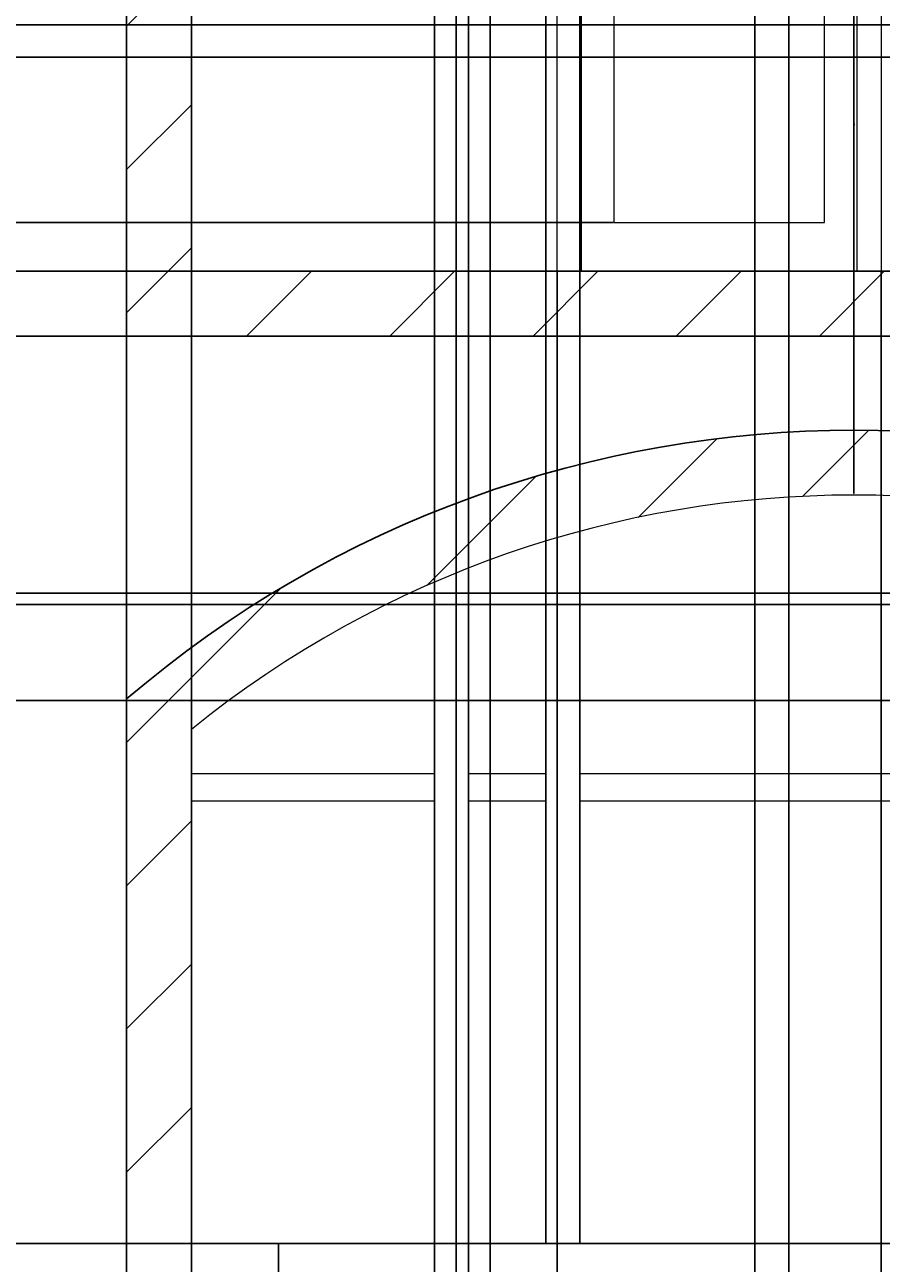
# Model space of a CAD drawing. Units: inches. Extents: x -14 to 375, y -86 to 549.
# Tile 3 of 12: x 122 to 227, y 4 to 156. Entities that reach past the tile are written whole.
import ezdxf

# ---------------------------------------------------------------- set-up
doc = ezdxf.new("R2010")
doc.units = ezdxf.units.IN
doc.header["$MEASUREMENT"] = 0
for name, color, linetype, lineweight in [('A-ANNO-DIMS', 2, 'Continuous', 18), ('A-DOOR', 3, 'Continuous', 18), ('A-ELEV', 7, 'Continuous', 25), ('A-ELEV-PATT', 8, 'Continuous', 13), ('A-GLAZ', 4, 'Continuous', 18)]:
    doc.layers.add(name, color=color, linetype=linetype, lineweight=lineweight)
doc.styles.get("Standard").update_dxf_attribs({"font": 'arial.ttf'})
doc.dimstyles.get("Standard").update_dxf_attribs({"dimtxt": 0.18, "dimasz": 0.18, "dimexe": 0.18, "dimexo": 0.0625, "dimgap": 0.09, "dimtad": 0, "dimtih": 1, "dimtoh": 1, "dimdec": 4, "dimzin": 0, "dimdsep": 46, "dimtxsty": 'Standard', "dimcen": 0.09, "dimadec": 0, "dimazin": 0, "dimtfac": 1, "dimtdec": 4, "dimtofl": 0, "dimtmove": 0, "dimatfit": 3, "dimfxl": 1, "dimtolj": 1, "dimtzin": 0, "dimarcsym": 0})

# ---------------------------------------------------------------- blocks, each defined once
blk = doc.blocks.new('*U3')
blk.add_lwpolyline([(3.12, 0.01), (0.12, 0.01), (0.12, 84.01), (40.12, 84.01), (40.12, 0.01), (37.12, 0.01)])
for points in [[(37.12, 80.99), (37.12, 0.01), (3.12, 0.01), (3.12, 80.99)], [(33.12, 6.01), (33.12, 74.99), (7.12, 74.99), (7.12, 6.01)]]:
    blk.add_lwpolyline(points, close=True)
blk.add_circle((35.12, 42.01), 1)
blk = doc.blocks.new('*D13')
at = {"layer": 'A-ANNO-DIMS', "color": 0, "lineweight": -2, "transparency": 16777216}
for p, q in [((134.17, 117.96), (-13.88, 117.96)), ((-13.7, 117.78), (-13.7, 95.65)), ((-13.7, 73.15), (-13.7, 95.28)), ((38.44, 72.97), (-13.88, 72.97))]:
    blk.add_line(p, q, dxfattribs=at)
at = {"layer": 'A-ANNO-DIMS', "color": 0, "transparency": 16777216}
for points in [[(-13.73, 117.78), (-13.67, 117.78), (-13.7, 117.96)], [(-13.73, 73.15), (-13.67, 73.15), (-13.7, 72.97)]]:
    blk.add_solid(points, dxfattribs=at)
at = {"layer": 'Defpoints', "color": 0, "transparency": 16777216}
for p in [(-13.7, 117.96), (134.23, 117.96), (38.5, 72.97)]:
    blk.add_point(p, dxfattribs=at)
at = {"layer": 'A-ANNO-DIMS', "color": 0, "transparency": 16777216, "insert": (-13.7, 95.46), "char_height": 0.18, "attachment_point": 5}
blk.add_mtext('\\A1;44.99', dxfattribs=at)
blk = doc.blocks.new('*D14')
at = {"layer": 'A-ANNO-DIMS', "color": 0, "lineweight": -2, "transparency": 16777216}
for p, q in [((38.44, 152.38), (-13.88, 152.38)), ((-13.7, 152.2), (-13.7, 135.35)), ((-13.7, 118.14), (-13.7, 134.99)), ((134.17, 117.96), (-13.88, 117.96))]:
    blk.add_line(p, q, dxfattribs=at)
at = {"layer": 'A-ANNO-DIMS', "color": 0, "transparency": 16777216}
for points in [[(-13.73, 152.2), (-13.67, 152.2), (-13.7, 152.38)], [(-13.73, 118.14), (-13.67, 118.14), (-13.7, 117.96)]]:
    blk.add_solid(points, dxfattribs=at)
at = {"layer": 'Defpoints', "color": 0, "transparency": 16777216}
for p in [(-13.7, 152.38), (38.5, 152.38), (134.23, 117.96)]:
    blk.add_point(p, dxfattribs=at)
at = {"layer": 'A-ANNO-DIMS', "color": 0, "transparency": 16777216, "insert": (-13.7, 135.17), "char_height": 0.18, "attachment_point": 5}
blk.add_mtext('\\A1;34.42', dxfattribs=at)
blk = doc.blocks.new('*D15')
at = {"layer": 'A-ANNO-DIMS', "color": 0, "lineweight": -2, "transparency": 16777216}
for p, q in [((134.17, 187.85), (-13.88, 187.85)), ((-13.7, 187.67), (-13.7, 170.29)), ((-13.7, 152.56), (-13.7, 169.93)), ((38.44, 152.38), (-13.88, 152.38))]:
    blk.add_line(p, q, dxfattribs=at)
at = {"layer": 'A-ANNO-DIMS', "color": 0, "transparency": 16777216}
for points in [[(-13.73, 187.67), (-13.67, 187.67), (-13.7, 187.85)], [(-13.73, 152.56), (-13.67, 152.56), (-13.7, 152.38)]]:
    blk.add_solid(points, dxfattribs=at)
at = {"layer": 'Defpoints', "color": 0, "transparency": 16777216}
for p in [(-13.7, 187.85), (134.23, 187.85), (38.5, 152.38)]:
    blk.add_point(p, dxfattribs=at)
at = {"layer": 'A-ANNO-DIMS', "color": 0, "transparency": 16777216, "insert": (-13.7, 170.11), "char_height": 0.18, "attachment_point": 5}
blk.add_mtext('\\A1;35.47', dxfattribs=at)
blk = doc.blocks.new('*D28')
at = {"layer": 'A-ANNO-DIMS', "color": 0, "lineweight": -2, "transparency": 16777216}
for p, q in [((107.764387, 156.376775), (374.544714, 156.376775)), ((374.364714, 156.196775), (374.364714, 154.556775)), ((374.364714, 152.556775), (374.364714, 154.196775)), ((111.764387, 152.376775), (374.544714, 152.376775))]:
    blk.add_line(p, q, dxfattribs=at)
at = {"layer": 'A-ANNO-DIMS', "color": 0, "transparency": 16777216}
for points in [[(374.334714, 156.196775), (374.394714, 156.196775), (374.364714, 156.376775)], [(374.334714, 152.556775), (374.394714, 152.556775), (374.364714, 152.376775)]]:
    blk.add_solid(points, dxfattribs=at)
at = {"layer": 'Defpoints', "color": 0, "transparency": 16777216}
for p in [(107.701887, 156.376775), (374.364714, 156.376775), (111.701887, 152.376775)]:
    blk.add_point(p, dxfattribs=at)
at = {"layer": 'A-ANNO-DIMS', "color": 0, "transparency": 16777216, "insert": (374.364714, 154.376775), "char_height": 0.18, "attachment_point": 5}
blk.add_mtext('\\A1;4', dxfattribs=at)
blk = doc.blocks.new('*D29')
at = {"layer": 'A-ANNO-DIMS', "color": 0, "lineweight": -2, "transparency": 16777216}
for p, q in [((107.74, 193.48), (374.54, 193.48)), ((374.36, 193.3), (374.36, 175.11)), ((374.36, 156.56), (374.36, 174.75)), ((107.76, 156.38), (374.54, 156.38))]:
    blk.add_line(p, q, dxfattribs=at)
at = {"layer": 'A-ANNO-DIMS', "color": 0, "transparency": 16777216}
for points in [[(374.33, 193.3), (374.39, 193.3), (374.36, 193.48)], [(374.33, 156.56), (374.39, 156.56), (374.36, 156.38)]]:
    blk.add_solid(points, dxfattribs=at)
at = {"layer": 'Defpoints', "color": 0, "transparency": 16777216}
for p in [(107.68, 193.48), (374.36, 193.48), (107.7, 156.38)]:
    blk.add_point(p, dxfattribs=at)
at = {"layer": 'A-ANNO-DIMS', "color": 0, "transparency": 16777216, "insert": (374.36, 174.93), "char_height": 0.18, "attachment_point": 5}
blk.add_mtext('\\A1;37.106', dxfattribs=at)
blk = doc.blocks.new('*D42')
at = {"layer": 'A-ANNO-DIMS', "color": 0, "lineweight": -2, "transparency": 16777216}
for p, q in [((142.23, 270.64), (142.23, -64.39)), ((134.23, 262.64), (134.23, -64.39)), ((134.41, -64.21), (138.08, -64.21)), ((142.05, -64.21), (138.38, -64.21))]:
    blk.add_line(p, q, dxfattribs=at)
at = {"layer": 'A-ANNO-DIMS', "color": 0, "transparency": 16777216}
for points in [[(134.41, -64.18), (134.41, -64.24), (134.23, -64.21)], [(142.05, -64.18), (142.05, -64.24), (142.23, -64.21)]]:
    blk.add_solid(points, dxfattribs=at)
at = {"layer": 'Defpoints', "color": 0, "transparency": 16777216}
for p in [(142.23, 270.71), (134.23, 262.71), (142.23, -64.21)]:
    blk.add_point(p, dxfattribs=at)
at = {"layer": 'A-ANNO-DIMS', "color": 0, "transparency": 16777216, "insert": (138.23, -64.21), "char_height": 0.18, "attachment_point": 5}
blk.add_mtext('\\A1;8', dxfattribs=at)
blk = doc.blocks.new('*D43')
at = {"layer": 'A-ANNO-DIMS', "color": 0, "lineweight": -2, "transparency": 16777216}
for p, q in [((142.23, 270.64), (142.23, -64.39)), ((305.63, 270.64), (305.63, -64.39)), ((142.41, -64.21), (223.55, -64.21)), ((305.45, -64.21), (224.32, -64.21))]:
    blk.add_line(p, q, dxfattribs=at)
at = {"layer": 'A-ANNO-DIMS', "color": 0, "transparency": 16777216}
for points in [[(142.41, -64.18), (142.41, -64.24), (142.23, -64.21)], [(305.45, -64.18), (305.45, -64.24), (305.63, -64.21)]]:
    blk.add_solid(points, dxfattribs=at)
at = {"layer": 'Defpoints', "color": 0, "transparency": 16777216}
for p in [(142.23, 270.71), (305.63, 270.71), (305.63, -64.21)]:
    blk.add_point(p, dxfattribs=at)
at = {"layer": 'A-ANNO-DIMS', "color": 0, "transparency": 16777216, "insert": (223.93, -64.21), "char_height": 0.18, "attachment_point": 5}
blk.add_mtext('\\A1;163.4', dxfattribs=at)
blk = doc.blocks.new('*D45')
at = {"layer": 'A-ANNO-DIMS', "color": 0, "lineweight": -2, "transparency": 16777216}
for p, q in [((142.23, 306.64), (142.23, -64.39)), ((174.92, 306.64), (174.92, -64.39)), ((142.41, -64.21), (158.19, -64.21)), ((174.74, -64.21), (158.97, -64.21))]:
    blk.add_line(p, q, dxfattribs=at)
at = {"layer": 'A-ANNO-DIMS', "color": 0, "transparency": 16777216}
for points in [[(142.41, -64.18), (142.41, -64.24), (142.23, -64.21)], [(174.74, -64.18), (174.74, -64.24), (174.92, -64.21)]]:
    blk.add_solid(points, dxfattribs=at)
at = {"layer": 'Defpoints', "color": 0, "transparency": 16777216}
for p in [(142.23, 306.71), (174.92, 306.71), (174.92, -64.21)]:
    blk.add_point(p, dxfattribs=at)
at = {"layer": 'A-ANNO-DIMS', "color": 0, "transparency": 16777216, "insert": (158.58, -64.21), "char_height": 0.18, "attachment_point": 5}
blk.add_mtext('\\A1;32.69', dxfattribs=at)
blk = doc.blocks.new('*D46')
at = {"layer": 'A-ANNO-DIMS', "color": 0, "lineweight": -2, "transparency": 16777216}
for p, q in [((174.92, 306.64), (174.92, -64.39)), ((179.09, 306.64), (179.09, -64.39)), ((175.1, -64.21), (176.68, -64.21)), ((178.91, -64.21), (177.33, -64.21))]:
    blk.add_line(p, q, dxfattribs=at)
at = {"layer": 'A-ANNO-DIMS', "color": 0, "transparency": 16777216}
for points in [[(175.1, -64.18), (175.1, -64.24), (174.92, -64.21)], [(178.91, -64.18), (178.91, -64.24), (179.09, -64.21)]]:
    blk.add_solid(points, dxfattribs=at)
at = {"layer": 'Defpoints', "color": 0, "transparency": 16777216}
for p in [(174.92, 306.71), (179.09, 306.71), (179.09, -64.21)]:
    blk.add_point(p, dxfattribs=at)
at = {"layer": 'A-ANNO-DIMS', "color": 0, "transparency": 16777216, "insert": (177.01, -64.21), "char_height": 0.18, "attachment_point": 5}
blk.add_mtext('\\A1;4.17', dxfattribs=at)
blk = doc.blocks.new('*D47')
at = {"layer": 'A-ANNO-DIMS', "color": 0, "lineweight": -2, "transparency": 16777216}
for p, q in [((179.09, 306.64), (179.09, -64.39)), ((211.78, 306.64), (211.78, -64.39)), ((179.27, -64.21), (195.04, -64.21)), ((211.6, -64.21), (195.83, -64.21))]:
    blk.add_line(p, q, dxfattribs=at)
at = {"layer": 'A-ANNO-DIMS', "color": 0, "transparency": 16777216}
for points in [[(179.27, -64.18), (179.27, -64.24), (179.09, -64.21)], [(211.6, -64.18), (211.6, -64.24), (211.78, -64.21)]]:
    blk.add_solid(points, dxfattribs=at)
at = {"layer": 'Defpoints', "color": 0, "transparency": 16777216}
for p in [(179.09, 306.71), (211.78, 306.71), (211.78, -64.21)]:
    blk.add_point(p, dxfattribs=at)
at = {"layer": 'A-ANNO-DIMS', "color": 0, "transparency": 16777216, "insert": (195.44, -64.21), "char_height": 0.18, "attachment_point": 5}
blk.add_mtext('\\A1;32.69', dxfattribs=at)
blk = doc.blocks.new('*D48')
at = {"layer": 'A-ANNO-DIMS', "color": 0, "lineweight": -2, "transparency": 16777216}
for p, q in [((211.78, 306.64), (211.78, -64.39)), ((215.95, 306.64), (215.95, -64.39)), ((211.96, -64.21), (213.54, -64.21)), ((215.77, -64.21), (214.19, -64.21))]:
    blk.add_line(p, q, dxfattribs=at)
at = {"layer": 'A-ANNO-DIMS', "color": 0, "transparency": 16777216}
for points in [[(211.96, -64.18), (211.96, -64.24), (211.78, -64.21)], [(215.77, -64.18), (215.77, -64.24), (215.95, -64.21)]]:
    blk.add_solid(points, dxfattribs=at)
at = {"layer": 'Defpoints', "color": 0, "transparency": 16777216}
for p in [(211.78, 306.71), (215.95, 306.71), (215.95, -64.21)]:
    blk.add_point(p, dxfattribs=at)
at = {"layer": 'A-ANNO-DIMS', "color": 0, "transparency": 16777216, "insert": (213.86, -64.21), "char_height": 0.18, "attachment_point": 5}
blk.add_mtext('\\A1;4.17', dxfattribs=at)
blk = doc.blocks.new('*D49')
at = {"layer": 'A-ANNO-DIMS', "color": 0, "lineweight": -2, "transparency": 16777216}
for p, q in [((215.95, 306.64), (215.95, -64.39)), ((248.64, 306.64), (248.64, -64.39)), ((216.13, -64.21), (231.9, -64.21)), ((248.46, -64.21), (232.69, -64.21))]:
    blk.add_line(p, q, dxfattribs=at)
at = {"layer": 'A-ANNO-DIMS', "color": 0, "transparency": 16777216}
for points in [[(216.13, -64.18), (216.13, -64.24), (215.95, -64.21)], [(248.46, -64.18), (248.46, -64.24), (248.64, -64.21)]]:
    blk.add_solid(points, dxfattribs=at)
at = {"layer": 'Defpoints', "color": 0, "transparency": 16777216}
for p in [(215.95, 306.71), (248.64, 306.71), (248.64, -64.21)]:
    blk.add_point(p, dxfattribs=at)
at = {"layer": 'A-ANNO-DIMS', "color": 0, "transparency": 16777216, "insert": (232.29, -64.21), "char_height": 0.18, "attachment_point": 5}
blk.add_mtext('\\A1;32.69', dxfattribs=at)
blk = doc.blocks.new('*D74')
at = {"layer": 'A-ANNO-DIMS', "color": 0, "lineweight": -2, "transparency": 16777216}
for p, q in [((142.23, 125.9), (142.23, -64.39)), ((134.23, 117.9), (134.23, -64.39)), ((134.41, -64.21), (138.08, -64.21)), ((142.05, -64.21), (138.38, -64.21))]:
    blk.add_line(p, q, dxfattribs=at)
at = {"layer": 'A-ANNO-DIMS', "color": 0, "transparency": 16777216}
for points in [[(134.41, -64.18), (134.41, -64.24), (134.23, -64.21)], [(142.05, -64.18), (142.05, -64.24), (142.23, -64.21)]]:
    blk.add_solid(points, dxfattribs=at)
at = {"layer": 'Defpoints', "color": 0, "transparency": 16777216}
for p in [(142.23, 125.96), (134.23, 117.96), (142.23, -64.21)]:
    blk.add_point(p, dxfattribs=at)
at = {"layer": 'A-ANNO-DIMS', "color": 0, "transparency": 16777216, "insert": (138.23, -64.21), "char_height": 0.18, "attachment_point": 5}
blk.add_mtext('\\A1;8', dxfattribs=at)
blk = doc.blocks.new('*D75')
at = {"layer": 'A-ANNO-DIMS', "color": 0, "lineweight": -2, "transparency": 16777216}
for p, q in [((142.23, 125.9), (142.23, -64.39)), ((172.23, 125.9), (172.23, -64.39)), ((142.41, -64.21), (157.01, -64.21)), ((172.05, -64.21), (157.45, -64.21))]:
    blk.add_line(p, q, dxfattribs=at)
at = {"layer": 'A-ANNO-DIMS', "color": 0, "transparency": 16777216}
for points in [[(142.41, -64.18), (142.41, -64.24), (142.23, -64.21)], [(172.05, -64.18), (172.05, -64.24), (172.23, -64.21)]]:
    blk.add_solid(points, dxfattribs=at)
at = {"layer": 'Defpoints', "color": 0, "transparency": 16777216}
for p in [(142.23, 125.96), (172.23, 125.96), (172.23, -64.21)]:
    blk.add_point(p, dxfattribs=at)
at = {"layer": 'A-ANNO-DIMS', "color": 0, "transparency": 16777216, "insert": (157.23, -64.21), "char_height": 0.18, "attachment_point": 5}
blk.add_mtext('\\A1;30', dxfattribs=at)
blk = doc.blocks.new('*D76')
at = {"layer": 'A-ANNO-DIMS', "color": 0, "lineweight": -2, "transparency": 16777216}
for p, q in [((172.23, 125.9), (172.23, -64.39)), ((176.42, 125.9), (176.42, -64.39)), ((172.41, -64.21), (173.93, -64.21)), ((176.24, -64.21), (174.72, -64.21))]:
    blk.add_line(p, q, dxfattribs=at)
at = {"layer": 'A-ANNO-DIMS', "color": 0, "transparency": 16777216}
for points in [[(172.41, -64.18), (172.41, -64.24), (172.23, -64.21)], [(176.24, -64.18), (176.24, -64.24), (176.42, -64.21)]]:
    blk.add_solid(points, dxfattribs=at)
at = {"layer": 'Defpoints', "color": 0, "transparency": 16777216}
for p in [(172.23, 125.96), (176.42, 125.96), (176.42, -64.21)]:
    blk.add_point(p, dxfattribs=at)
at = {"layer": 'A-ANNO-DIMS', "color": 0, "transparency": 16777216, "insert": (174.32, -64.21), "char_height": 0.18, "attachment_point": 5}
blk.add_mtext('\\A1;4.186', dxfattribs=at)
blk = doc.blocks.new('*D77')
at = {"layer": 'A-ANNO-DIMS', "color": 0, "lineweight": -2, "transparency": 16777216}
for p, q in [((176.42, 125.9), (176.42, -64.39)), ((187.37, 125.91), (187.37, -64.39)), ((176.6, -64.21), (181.44, -64.21)), ((187.19, -64.21), (182.35, -64.21))]:
    blk.add_line(p, q, dxfattribs=at)
at = {"layer": 'A-ANNO-DIMS', "color": 0, "transparency": 16777216}
for points in [[(176.6, -64.18), (176.6, -64.24), (176.42, -64.21)], [(187.19, -64.18), (187.19, -64.24), (187.37, -64.21)]]:
    blk.add_solid(points, dxfattribs=at)
at = {"layer": 'Defpoints', "color": 0, "transparency": 16777216}
for p in [(176.42, 125.96), (187.37, 125.97), (187.37, -64.21)]:
    blk.add_point(p, dxfattribs=at)
at = {"layer": 'A-ANNO-DIMS', "color": 0, "transparency": 16777216, "insert": (181.89, -64.21), "char_height": 0.18, "attachment_point": 5}
blk.add_mtext('\\A1;10.949', dxfattribs=at)
blk = doc.blocks.new('*D78')
at = {"layer": 'A-ANNO-DIMS', "color": 0, "lineweight": -2, "transparency": 16777216}
for p, q in [((187.37, 125.91), (187.37, -64.39)), ((227.37, 125.91), (227.37, -64.39)), ((187.55, -64.21), (207.14, -64.21)), ((227.19, -64.21), (207.59, -64.21))]:
    blk.add_line(p, q, dxfattribs=at)
at = {"layer": 'A-ANNO-DIMS', "color": 0, "transparency": 16777216}
for points in [[(187.55, -64.18), (187.55, -64.24), (187.37, -64.21)], [(227.19, -64.18), (227.19, -64.24), (227.37, -64.21)]]:
    blk.add_solid(points, dxfattribs=at)
at = {"layer": 'Defpoints', "color": 0, "transparency": 16777216}
for p in [(187.37, 125.97), (227.37, 125.97), (227.37, -64.21)]:
    blk.add_point(p, dxfattribs=at)
at = {"layer": 'A-ANNO-DIMS', "color": 0, "transparency": 16777216, "insert": (207.37, -64.21), "char_height": 0.18, "attachment_point": 5}
blk.add_mtext('\\A1;40', dxfattribs=at)
blk = doc.blocks.new('*D95')
at = {"layer": 'A-ANNO-DIMS', "color": 0, "lineweight": -2, "transparency": 16777216}
for p, q in [((194.3, 131.97), (-13.88, 131.97)), ((-13.7, 131.79), (-13.7, 129.15)), ((-13.7, 126.15), (-13.7, 128.79)), ((187.3, 125.97), (-13.88, 125.97))]:
    blk.add_line(p, q, dxfattribs=at)
at = {"layer": 'A-ANNO-DIMS', "color": 0, "transparency": 16777216}
for points in [[(-13.73, 131.79), (-13.67, 131.79), (-13.7, 131.97)], [(-13.73, 126.15), (-13.67, 126.15), (-13.7, 125.97)]]:
    blk.add_solid(points, dxfattribs=at)
at = {"layer": 'Defpoints', "color": 0, "transparency": 16777216}
for p in [(-13.7, 131.97), (194.37, 131.97), (187.37, 125.97)]:
    blk.add_point(p, dxfattribs=at)
at = {"layer": 'A-ANNO-DIMS', "color": 0, "transparency": 16777216, "insert": (-13.7, 128.97), "char_height": 0.18, "attachment_point": 5}
blk.add_mtext('\\A1;6', dxfattribs=at)
blk = doc.blocks.new('*D96')
at = {"layer": 'A-ANNO-DIMS', "color": 0, "lineweight": -2, "transparency": 16777216}
for p, q in [((194.3, 200.95), (-13.88, 200.95)), ((-13.7, 200.77), (-13.7, 166.64)), ((-13.7, 132.15), (-13.7, 166.28)), ((194.3, 131.97), (-13.88, 131.97))]:
    blk.add_line(p, q, dxfattribs=at)
at = {"layer": 'A-ANNO-DIMS', "color": 0, "transparency": 16777216}
for points in [[(-13.73, 200.77), (-13.67, 200.77), (-13.7, 200.95)], [(-13.73, 132.15), (-13.67, 132.15), (-13.7, 131.97)]]:
    blk.add_solid(points, dxfattribs=at)
at = {"layer": 'Defpoints', "color": 0, "transparency": 16777216}
for p in [(-13.7, 200.95), (194.37, 200.95), (194.37, 131.97)]:
    blk.add_point(p, dxfattribs=at)
at = {"layer": 'A-ANNO-DIMS', "color": 0, "transparency": 16777216, "insert": (-13.7, 166.46), "char_height": 0.18, "attachment_point": 5}
blk.add_mtext('\\A1;68.98', dxfattribs=at)
blk = doc.blocks.new('*D99')
at = {"layer": 'A-ANNO-DIMS', "color": 0, "lineweight": -2, "transparency": 16777216}
for p, q in [((134.23, 6.02), (134.23, 515.24)), ((142.23, 6.02), (142.23, 515.24)), ((134.41, 515.06), (138.08, 515.06)), ((142.05, 515.06), (138.38, 515.06))]:
    blk.add_line(p, q, dxfattribs=at)
at = {"layer": 'A-ANNO-DIMS', "color": 0, "transparency": 16777216}
for points in [[(134.41, 515.09), (134.41, 515.03), (134.23, 515.06)], [(142.05, 515.09), (142.05, 515.03), (142.23, 515.06)]]:
    blk.add_solid(points, dxfattribs=at)
at = {"layer": 'Defpoints', "color": 0, "transparency": 16777216}
for p in [(142.23, 515.06), (134.23, 5.96), (142.23, 5.96)]:
    blk.add_point(p, dxfattribs=at)
at = {"layer": 'A-ANNO-DIMS', "color": 0, "transparency": 16777216, "insert": (138.23, 515.06), "char_height": 0.18, "attachment_point": 5}
blk.add_mtext('\\A1;8', dxfattribs=at)
blk = doc.blocks.new('*D100')
at = {"layer": 'A-ANNO-DIMS', "color": 0, "lineweight": -2, "transparency": 16777216}
for p, q in [((142.23, 6.02), (142.23, 515.24)), ((172.23, 6.02), (172.23, 515.24)), ((142.41, 515.06), (157.01, 515.06)), ((172.05, 515.06), (157.45, 515.06))]:
    blk.add_line(p, q, dxfattribs=at)
at = {"layer": 'A-ANNO-DIMS', "color": 0, "transparency": 16777216}
for points in [[(142.41, 515.09), (142.41, 515.03), (142.23, 515.06)], [(172.05, 515.09), (172.05, 515.03), (172.23, 515.06)]]:
    blk.add_solid(points, dxfattribs=at)
at = {"layer": 'Defpoints', "color": 0, "transparency": 16777216}
for p in [(172.23, 515.06), (142.23, 5.96), (172.23, 5.96)]:
    blk.add_point(p, dxfattribs=at)
at = {"layer": 'A-ANNO-DIMS', "color": 0, "transparency": 16777216, "insert": (157.23, 515.06), "char_height": 0.18, "attachment_point": 5}
blk.add_mtext('\\A1;30', dxfattribs=at)
blk = doc.blocks.new('*D101')
at = {"layer": 'A-ANNO-DIMS', "color": 0, "lineweight": -2, "transparency": 16777216}
for p, q in [((172.23, 6.02), (172.23, 515.24)), ((176.42, 6.02), (176.42, 515.24)), ((172.41, 515.06), (173.93, 515.06)), ((176.24, 515.06), (174.72, 515.06))]:
    blk.add_line(p, q, dxfattribs=at)
at = {"layer": 'A-ANNO-DIMS', "color": 0, "transparency": 16777216}
for points in [[(172.41, 515.09), (172.41, 515.03), (172.23, 515.06)], [(176.24, 515.09), (176.24, 515.03), (176.42, 515.06)]]:
    blk.add_solid(points, dxfattribs=at)
at = {"layer": 'Defpoints', "color": 0, "transparency": 16777216}
for p in [(176.42, 515.06), (172.23, 5.96), (176.42, 5.96)]:
    blk.add_point(p, dxfattribs=at)
at = {"layer": 'A-ANNO-DIMS', "color": 0, "transparency": 16777216, "insert": (174.32, 515.06), "char_height": 0.18, "attachment_point": 5}
blk.add_mtext('\\A1;4.186', dxfattribs=at)
blk = doc.blocks.new('*D102')
at = {"layer": 'A-ANNO-DIMS', "color": 0, "lineweight": -2, "transparency": 16777216}
for p, q in [((176.42, 6.02), (176.42, 515.24)), ((185.96, 6.02), (185.96, 515.24)), ((176.6, 515.06), (180.8, 515.06)), ((185.78, 515.06), (181.58, 515.06))]:
    blk.add_line(p, q, dxfattribs=at)
at = {"layer": 'A-ANNO-DIMS', "color": 0, "transparency": 16777216}
for points in [[(176.6, 515.09), (176.6, 515.03), (176.42, 515.06)], [(185.78, 515.09), (185.78, 515.03), (185.96, 515.06)]]:
    blk.add_solid(points, dxfattribs=at)
at = {"layer": 'Defpoints', "color": 0, "transparency": 16777216}
for p in [(185.96, 515.06), (176.42, 5.96), (185.96, 5.96)]:
    blk.add_point(p, dxfattribs=at)
at = {"layer": 'A-ANNO-DIMS', "color": 0, "transparency": 16777216, "insert": (181.19, 515.06), "char_height": 0.18, "attachment_point": 5}
blk.add_mtext('\\A1;9.545', dxfattribs=at)
blk = doc.blocks.new('*D103')
at = {"layer": 'A-ANNO-DIMS', "color": 0, "lineweight": -2, "transparency": 16777216}
for p, q in [((185.96, 6.02), (185.96, 515.24)), ((190.15, 6.02), (190.15, 515.24)), ((186.14, 515.06), (187.66, 515.06)), ((189.97, 515.06), (188.45, 515.06))]:
    blk.add_line(p, q, dxfattribs=at)
at = {"layer": 'A-ANNO-DIMS', "color": 0, "transparency": 16777216}
for points in [[(186.14, 515.09), (186.14, 515.03), (185.96, 515.06)], [(189.97, 515.09), (189.97, 515.03), (190.15, 515.06)]]:
    blk.add_solid(points, dxfattribs=at)
at = {"layer": 'Defpoints', "color": 0, "transparency": 16777216}
for p in [(190.15, 515.06), (185.96, 5.96), (190.15, 5.96)]:
    blk.add_point(p, dxfattribs=at)
at = {"layer": 'A-ANNO-DIMS', "color": 0, "transparency": 16777216, "insert": (188.06, 515.06), "char_height": 0.18, "attachment_point": 5}
blk.add_mtext('\\A1;4.186', dxfattribs=at)
blk = doc.blocks.new('*D104')
at = {"layer": 'A-ANNO-DIMS', "color": 0, "lineweight": -2, "transparency": 16777216}
for p, q in [((190.15, 6.02), (190.15, 515.24)), ((271, 6.02), (271, 515.24)), ((190.33, 515.06), (230.18, 515.06)), ((270.82, 515.06), (230.97, 515.06))]:
    blk.add_line(p, q, dxfattribs=at)
at = {"layer": 'A-ANNO-DIMS', "color": 0, "transparency": 16777216}
for points in [[(190.33, 515.09), (190.33, 515.03), (190.15, 515.06)], [(270.82, 515.09), (270.82, 515.03), (271, 515.06)]]:
    blk.add_solid(points, dxfattribs=at)
at = {"layer": 'Defpoints', "color": 0, "transparency": 16777216}
for p in [(271, 515.06), (190.15, 5.96), (271, 5.96)]:
    blk.add_point(p, dxfattribs=at)
at = {"layer": 'A-ANNO-DIMS', "color": 0, "transparency": 16777216, "insert": (230.57, 515.06), "char_height": 0.18, "attachment_point": 5}
blk.add_mtext('\\A1;80.85', dxfattribs=at)
blk = doc.blocks.new('*D108')
at = {"layer": 'A-ANNO-DIMS', "color": 0, "lineweight": -2, "transparency": 16777216}
for p, q in [((134.23, 5.9), (134.23, -64.39)), ((152.96, -7.79), (152.96, -64.39)), ((134.41, -64.21), (143.21, -64.21)), ((152.78, -64.21), (143.98, -64.21))]:
    blk.add_line(p, q, dxfattribs=at)
at = {"layer": 'A-ANNO-DIMS', "color": 0, "transparency": 16777216}
for points in [[(134.41, -64.18), (134.41, -64.24), (134.23, -64.21)], [(152.78, -64.18), (152.78, -64.24), (152.96, -64.21)]]:
    blk.add_solid(points, dxfattribs=at)
at = {"layer": 'Defpoints', "color": 0, "transparency": 16777216}
for p in [(134.23, 5.96), (152.96, -7.73), (152.96, -64.21)]:
    blk.add_point(p, dxfattribs=at)
at = {"layer": 'A-ANNO-DIMS', "color": 0, "transparency": 16777216, "insert": (143.6, -64.21), "char_height": 0.18, "attachment_point": 5}
blk.add_mtext('\\A1;18.73', dxfattribs=at)
blk = doc.blocks.new('*D128')
at = {"layer": 'A-ANNO-DIMS', "color": 0, "lineweight": -2, "transparency": 16777216}
for p, q in [((96.79, 84.82), (374.54, 84.82)), ((374.36, 84.64), (374.36, 79.07)), ((374.36, 73.15), (374.36, 78.71)), ((111.56, 72.97), (374.54, 72.97))]:
    blk.add_line(p, q, dxfattribs=at)
at = {"layer": 'A-ANNO-DIMS', "color": 0, "transparency": 16777216}
for points in [[(374.33, 84.64), (374.39, 84.64), (374.36, 84.82)], [(374.33, 73.15), (374.39, 73.15), (374.36, 72.97)]]:
    blk.add_solid(points, dxfattribs=at)
at = {"layer": 'Defpoints', "color": 0, "transparency": 16777216}
for p in [(96.73, 84.82), (374.36, 84.82), (111.5, 72.97)]:
    blk.add_point(p, dxfattribs=at)
at = {"layer": 'A-ANNO-DIMS', "color": 0, "transparency": 16777216, "insert": (374.36, 78.89), "char_height": 0.18, "attachment_point": 5}
blk.add_mtext('\\A1;11.849', dxfattribs=at)
blk = doc.blocks.new('*D129')
at = {"layer": 'A-ANNO-DIMS', "color": 0, "lineweight": -2, "transparency": 16777216}
for p, q in [((96.79, 86.23), (374.54, 86.23)), ((374.36, 86.05), (374.36, 85.7)), ((96.79, 84.82), (374.54, 84.82)), ((374.36, 85), (374.36, 85.34))]:
    blk.add_line(p, q, dxfattribs=at)
at = {"layer": 'A-ANNO-DIMS', "color": 0, "transparency": 16777216}
for points in [[(374.33, 86.05), (374.39, 86.05), (374.36, 86.23)], [(374.33, 85), (374.39, 85), (374.36, 84.82)]]:
    blk.add_solid(points, dxfattribs=at)
at = {"layer": 'Defpoints', "color": 0, "transparency": 16777216}
for p in [(96.73, 86.23), (374.36, 86.23), (96.73, 84.82)]:
    blk.add_point(p, dxfattribs=at)
at = {"layer": 'A-ANNO-DIMS', "color": 0, "transparency": 16777216, "insert": (374.36, 85.52), "char_height": 0.18, "attachment_point": 5}
blk.add_mtext('\\A1;1.409', dxfattribs=at)
blk = doc.blocks.new('*D135')
at = {"layer": 'A-ANNO-DIMS', "color": 0, "lineweight": -2, "transparency": 16777216}
for p, q in [((224.18, 303.87), (224, 303.87)), ((224, 303.87), (224, 244.12)), ((223.91, 144.06), (224.09, 144.06)), ((224, 143.97), (224, 144.15))]:
    blk.add_line(p, q, dxfattribs=at)
at = {"layer": 'A-ANNO-DIMS', "color": 0, "transparency": 16777216}
blk.add_solid([(223.97, 244.12), (224.03, 244.12), (224, 243.94)], dxfattribs=at)
at = {"layer": 'Defpoints', "color": 0, "transparency": 16777216}
for p in [(224, 243.94), (224, 144.06)]:
    blk.add_point(p, dxfattribs=at)
at = {"layer": 'A-ANNO-DIMS', "color": 0, "transparency": 16777216, "insert": (224.66, 303.87), "char_height": 0.18, "attachment_point": 5}
blk.add_mtext('\\A1;R99.88', dxfattribs=at)
blk = doc.blocks.new('*D136')
at = {"layer": 'A-ANNO-DIMS', "color": 0, "lineweight": -2, "transparency": 16777216}
for p, q in [((224.18, 291.07), (224, 291.07)), ((224, 291.07), (224, 236.12)), ((223.91, 144.06), (224.09, 144.06)), ((224, 143.97), (224, 144.15))]:
    blk.add_line(p, q, dxfattribs=at)
at = {"layer": 'A-ANNO-DIMS', "color": 0, "transparency": 16777216}
blk.add_solid([(223.97, 236.12), (224.03, 236.12), (224, 235.94)], dxfattribs=at)
at = {"layer": 'Defpoints', "color": 0, "transparency": 16777216}
for p in [(224, 235.94), (224, 144.06)]:
    blk.add_point(p, dxfattribs=at)
at = {"layer": 'A-ANNO-DIMS', "color": 0, "transparency": 16777216, "insert": (224.66, 291.07), "char_height": 0.18, "attachment_point": 5}
blk.add_mtext('\\A1;R91.88', dxfattribs=at)
blk = doc.blocks.new('*D137')
at = {"layer": 'A-ANNO-DIMS', "color": 0, "lineweight": -2, "transparency": 16777216}
for p, q in [((224.18, 189.18), (224, 189.18)), ((224, 189.18), (224, 106.51)), ((223.91, -31.75), (224.09, -31.75)), ((224, -31.84), (224, -31.66))]:
    blk.add_line(p, q, dxfattribs=at)
at = {"layer": 'A-ANNO-DIMS', "color": 0, "transparency": 16777216}
blk.add_solid([(223.97, 106.51), (224.03, 106.51), (224, 106.33)], dxfattribs=at)
at = {"layer": 'Defpoints', "color": 0, "transparency": 16777216}
for p in [(224, 106.33), (224, -31.75)]:
    blk.add_point(p, dxfattribs=at)
at = {"layer": 'A-ANNO-DIMS', "color": 0, "transparency": 16777216, "insert": (224.73, 189.18), "char_height": 0.18, "attachment_point": 5}
blk.add_mtext('\\A1;R138.08', dxfattribs=at)
blk = doc.blocks.new('*D138')
at = {"layer": 'A-ANNO-DIMS', "color": 0, "lineweight": -2, "transparency": 16777216}
for p, q in [((224.18, 176.38), (224, 176.38)), ((224, 176.38), (224, 98.51)), ((223.91, -31.75), (224.09, -31.75)), ((224, -31.84), (224, -31.66))]:
    blk.add_line(p, q, dxfattribs=at)
at = {"layer": 'A-ANNO-DIMS', "color": 0, "transparency": 16777216}
blk.add_solid([(223.97, 98.51), (224.03, 98.51), (224, 98.33)], dxfattribs=at)
at = {"layer": 'Defpoints', "color": 0, "transparency": 16777216}
for p in [(224, 98.33), (224, -31.75)]:
    blk.add_point(p, dxfattribs=at)
at = {"layer": 'A-ANNO-DIMS', "color": 0, "transparency": 16777216, "insert": (224.73, 176.38), "char_height": 0.18, "attachment_point": 5}
blk.add_mtext('\\A1;R130.08', dxfattribs=at)

msp = doc.modelspace()

# ---------------------------------------------------------------- hatches: boundary and pattern name
at = {"layer": 'A-ELEV-PATT'}
h = msp.add_hatch(dxfattribs=at)
h.set_pattern_fill('ANSI31', color=256, scale=100)
h.set_pattern_definition([(45, (-168.406, -22.703), (-8.83883, 8.83883), [])])
h.paths.add_polyline_path([(313.6281, 262.7071), (313.6281, 357.9589), (313.7701, 357.9589), (313.7701, 433.1717, 0.36940998), (134.2334, 433.1717), (134.2334, 365.9589), (134.2334, 262.7071)])
h.paths.add_polyline_path([(142.2334, 270.7071), (142.2334, 365.9589), (142.2334, 429.4208, -0.35358711), (305.7701, 429.4208), (305.7701, 365.9589), (305.6281, 365.9589), (305.6281, 270.7071)], flags=16)
h.paths.add_polyline_path([(134.2334, 187.8466), (134.2334, 117.9589), (313.7701, 117.9589), (313.7701, 187.8466, 0.62486768)])
h.paths.add_polyline_path([(305.7701, 185.9589), (305.7701, 125.9589), (142.2334, 125.9589), (142.2334, 185.9589, -0.61125102)], flags=16)
h.paths.add_polyline_path([(134.2334, 73.1717), (134.2334, 5.9589), (142.2334, 5.9589), (142.2334, 69.4208, -0.35358711), (305.7701, 69.4208), (305.7701, 5.9589), (313.7701, 5.9589), (313.7701, 73.1717, 0.36940998)])

# ---------------------------------------------------------------- linework, layer by layer
at = {"layer": 'A-ELEV'}
msp.add_line((15.4018, 5.9589), (345.2647, 5.9589), dxfattribs=at)
for points in [[(134.2334, 187.8466), (134.2334, 117.9589), (313.7701, 117.9589), (313.7701, 187.8466, 0.62486768)], [(142.2334, 185.9589), (142.2334, 125.9589), (305.7701, 125.9589), (305.7701, 185.9589, 0.61125102)]]:
    msp.add_lwpolyline(points, format="xyb", close=True, dxfattribs=at)
msp.add_lwpolyline([(313.7701, 5.9589), (313.7701, 73.1717, 0.36940998), (134.2334, 73.1717), (134.2334, 5.9589)], format="xyb", dxfattribs=at)
for points in [[(15.4018, 5.9589), (345.2647, 5.9589), (345.2647, -35.1115), (15.4018, -35.1115)], [(152.9633, 5.9589), (297.193, 5.9589), (297.193, -7.7312), (152.9633, -7.7312)]]:
    msp.add_lwpolyline(points, close=True, dxfattribs=at)
at = {"layer": 'A-GLAZ'}
for points in [[(176.4171, 222.6573), (176.4171, 125.9589)], [(176.4171, 176.9318), (176.4171, 125.9589), (172.2314, 125.9589), (172.2314, 176.9318)], [(190.148, 93.8506), (190.148, 63.9218)], [(185.9623, 63.9218), (185.9623, 92.6469)], [(176.4171, 89.3173), (176.4171, 63.9218)], [(172.2314, 63.9218), (172.2314, 87.5874)], [(172.2314, 63.9218), (142.2334, 63.9218), (142.2334, 60.5886), (172.2314, 60.5886)], [(185.9623, 63.9218), (176.4171, 63.9218)], [(270.9993, 63.9218), (190.148, 63.9218)], [(176.4171, 60.5886), (176.4171, 5.9589), (172.2314, 5.9589), (172.2314, 60.5886)], [(176.4171, 60.5886), (185.9623, 60.5886)], [(190.148, 60.5886), (190.148, 5.9589), (185.9623, 5.9589), (185.9623, 60.5886)], [(190.148, 60.5886), (270.9993, 60.5886)]]:
    msp.add_lwpolyline(points, dxfattribs=at)
msp.add_lwpolyline([(305.7701, 5.9589), (305.7701, 69.4208, 0.35358711), (142.2334, 69.4208), (142.2334, 5.9589)], format="xyb", dxfattribs=at)

# ---------------------------------------------------------------- block references
at = {"layer": 'A-DOOR'}
msp.add_blockref('*U3', (187.242, 125.9589), dxfattribs=at)

# ---------------------------------------------------------------- dimensions: what is measured, and where the dimension line sits
at = {"layer": 'A-ANNO-DIMS'}
for base, p1, p2, override, picture, middle in [((142.2334, 515.0589), (134.2334, 5.9589), (142.2334, 5.9589), {"dimdec": 0, "dimlfac": 1, "dimrnd": 0, "dimzin": 0, "dimdsep": 46, "dimlunit": 2}, '*D99', (138.2334, 515.0589)), ((172.2314, 515.0589), (142.2334, 5.9589), (172.2314, 5.9589), {"dimdec": 0, "dimlfac": 1, "dimrnd": 0, "dimzin": 0, "dimdsep": 46, "dimlunit": 2}, '*D100', (157.2324, 515.0589)), ((176.4171, 515.0589), (172.2314, 5.9589), (176.4171, 5.9589), {"dimdec": 3, "dimlfac": 1, "dimrnd": 0, "dimzin": 0, "dimdsep": 46, "dimlunit": 2}, '*D101', (174.3243, 515.0589)), ((185.9623, 515.0589), (176.4171, 5.9589), (185.9623, 5.9589), {"dimdec": 3, "dimlfac": 1, "dimrnd": 0, "dimzin": 0, "dimdsep": 46, "dimlunit": 2}, '*D102', (181.1897, 515.0589)), ((190.148, 515.0589), (185.9623, 5.9589), (190.148, 5.9589), {"dimdec": 3, "dimlfac": 1, "dimrnd": 0, "dimzin": 0, "dimdsep": 46, "dimlunit": 2}, '*D103', (188.0551, 515.0589)), ((270.9993, 515.0589), (190.148, 5.9589), (270.9993, 5.9589), {"dimdec": 2, "dimlfac": 1, "dimrnd": 0, "dimzin": 0, "dimdsep": 46, "dimlunit": 2}, '*D104', (230.5736, 515.0589)), ((174.9243, -64.2115), (142.2334, 306.7071), (174.9243, 306.7071), {"dimdec": 2, "dimlfac": 1, "dimrnd": 0, "dimzin": 0, "dimdsep": 46, "dimlunit": 2}, '*D45', (158.5788, -64.2115)), ((179.0907, -64.2115), (174.9243, 306.7071), (179.0907, 306.7071), {"dimdec": 2, "dimlfac": 1, "dimrnd": 0, "dimzin": 0, "dimdsep": 46, "dimlunit": 2}, '*D46', (177.0075, -64.2115)), ((211.7816, -64.2115), (179.0907, 306.7071), (211.7816, 306.7071), {"dimdec": 2, "dimlfac": 1, "dimrnd": 0, "dimzin": 0, "dimdsep": 46, "dimlunit": 2}, '*D47', (195.4362, -64.2115)), ((215.9481, -64.2115), (211.7816, 306.7071), (215.9481, 306.7071), {"dimdec": 2, "dimlfac": 1, "dimrnd": 0, "dimzin": 0, "dimdsep": 46, "dimlunit": 2}, '*D48', (213.8649, -64.2115)), ((248.639, -64.2115), (215.9481, 306.7071), (248.639, 306.7071), {"dimdec": 2, "dimlfac": 1, "dimrnd": 0, "dimzin": 0, "dimdsep": 46, "dimlunit": 2}, '*D49', (232.2936, -64.2115)), ((142.2334, -64.2115), (134.2334, 262.7071), (142.2334, 270.7071), {"dimdec": 0, "dimlfac": 1, "dimrnd": 0, "dimzin": 0, "dimdsep": 46, "dimlunit": 2}, '*D42', (138.2334, -64.2115)), ((305.6281, -64.2115), (142.2334, 270.7071), (305.6281, 270.7071), {"dimdec": 1, "dimlfac": 1, "dimrnd": 0, "dimzin": 0, "dimdsep": 46, "dimlunit": 2}, '*D43', (223.9307, -64.2115)), ((142.2334, -64.2115), (134.2334, 117.9589), (142.2334, 125.9589), {"dimdec": 0, "dimlfac": 1, "dimrnd": 0, "dimzin": 0, "dimdsep": 46, "dimlunit": 2}, '*D74', (138.2334, -64.2115)), ((172.2314, -64.2115), (142.2334, 125.9589), (172.2314, 125.9589), {"dimdec": 0, "dimlfac": 1, "dimrnd": 0, "dimzin": 0, "dimdsep": 46, "dimlunit": 2}, '*D75', (157.2324, -64.2115)), ((176.4171, -64.2115), (172.2314, 125.9589), (176.4171, 125.9589), {"dimdec": 3, "dimlfac": 1, "dimrnd": 0, "dimzin": 0, "dimdsep": 46, "dimlunit": 2}, '*D76', (174.3243, -64.2115)), ((187.3657, -64.2115), (176.4171, 125.9589), (187.3657, 125.9717), {"dimdec": 3, "dimlfac": 1, "dimrnd": 0, "dimzin": 0, "dimdsep": 46, "dimlunit": 2}, '*D77', (181.8914, -64.2115)), ((227.3657, -64.2115), (187.3657, 125.9717), (227.3657, 125.9717), {"dimdec": 0, "dimlfac": 1, "dimrnd": 0, "dimzin": 0, "dimdsep": 46, "dimlunit": 2}, '*D78', (207.3657, -64.2115)), ((152.9633, -64.2115), (134.2334, 5.9589), (152.9633, -7.7312), {"dimdec": 2, "dimlfac": 1, "dimrnd": 0, "dimzin": 0, "dimdsep": 46, "dimlunit": 2}, '*D108', (143.5984, -64.2115))]:
    dim = msp.add_linear_dim(base=base, p1=p1, p2=p2, dimstyle='Standard', override=override, dxfattribs=at)
    dim.commit()
    dim.dimension.update_dxf_attribs({"geometry": picture, "text_midpoint": middle})
for center, mpoint, picture, middle in [((224.0017, 144.0634), (224.002, 243.9399), '*D135', (224.6622, 303.8658)), ((224.0017, 144.0634), (224.002, 235.9399), '*D136', (224.6622, 291.0658)), ((224.0017, -31.75), (224.002, 106.333), '*D137', (224.7321, 189.1828)), ((224.0017, -31.75), (224.002, 98.333), '*D138', (224.7321, 176.3828))]:
    dim = msp.add_radius_dim(center=center, mpoint=mpoint, dimstyle='Standard', override={"dimdec": 2, "dimlfac": 1, "dimrnd": 0, "dimzin": 0, "dimdsep": 46, "dimlunit": 2}, dxfattribs=at)
    dim.commit()
    dim.dimension.update_dxf_attribs({"geometry": picture, "text_midpoint": middle, "dimtype": 164})
for base, p1, p2, override, picture, middle in [((-13.6982, 200.9487), (194.3657, 131.9717), (194.3657, 200.9487), {"dimdec": 2, "dimlfac": 1, "dimrnd": 0, "dimzin": 0, "dimdsep": 46, "dimlunit": 2}, '*D96', (-13.6982, 166.4602)), ((374.3647, 193.4825), (107.7019, 156.3768), (107.6798, 193.4825), {"dimdec": 3, "dimlfac": 1, "dimrnd": 0, "dimzin": 0, "dimdsep": 46, "dimlunit": 2}, '*D29', (374.3647, 174.9296)), ((-13.6982, 187.8466), (38.5033, 152.3768), (134.2334, 187.8466), {"dimdec": 2, "dimlfac": 1, "dimrnd": 0, "dimzin": 0, "dimdsep": 46, "dimlunit": 2}, '*D15', (-13.6982, 170.1117)), ((374.3647, 156.3768), (111.7019, 152.3768), (107.7019, 156.3768), {"dimdec": 0, "dimlfac": 1, "dimrnd": 0, "dimzin": 0, "dimdsep": 46, "dimlunit": 2}, '*D28', (374.3647, 154.3768)), ((-13.6982, 152.3768), (134.2334, 117.9589), (38.5033, 152.3768), {"dimdec": 2, "dimlfac": 1, "dimrnd": 0, "dimzin": 0, "dimdsep": 46, "dimlunit": 2}, '*D14', (-13.6982, 135.1678)), ((-13.6982, 131.9717), (187.3657, 125.9717), (194.3657, 131.9717), {"dimdec": 0, "dimlfac": 1, "dimrnd": 0, "dimzin": 0, "dimdsep": 46, "dimlunit": 2}, '*D95', (-13.6982, 128.9717)), ((-13.6982, 117.9589), (38.5033, 72.9679), (134.2334, 117.9589), {"dimdec": 2, "dimlfac": 1, "dimrnd": 0, "dimzin": 0, "dimdsep": 46, "dimlunit": 2}, '*D13', (-13.6982, 95.4634)), ((374.3647, 86.2255), (96.7255, 84.8165), (96.7255, 86.2255), {"dimdec": 3, "dimlfac": 1, "dimrnd": 0, "dimzin": 0, "dimdsep": 46, "dimlunit": 2}, '*D129', (374.3647, 85.521)), ((374.3647, 84.8165), (111.4987, 72.9679), (96.7255, 84.8165), {"dimdec": 3, "dimlfac": 1, "dimrnd": 0, "dimzin": 0, "dimdsep": 46, "dimlunit": 2}, '*D128', (374.3647, 78.8922))]:
    dim = msp.add_linear_dim(base=base, p1=p1, p2=p2, angle=90, dimstyle='Standard', override=override, dxfattribs=at)
    dim.commit()
    dim.dimension.update_dxf_attribs({"geometry": picture, "text_midpoint": middle})

doc.saveas('drawing.dxf')
